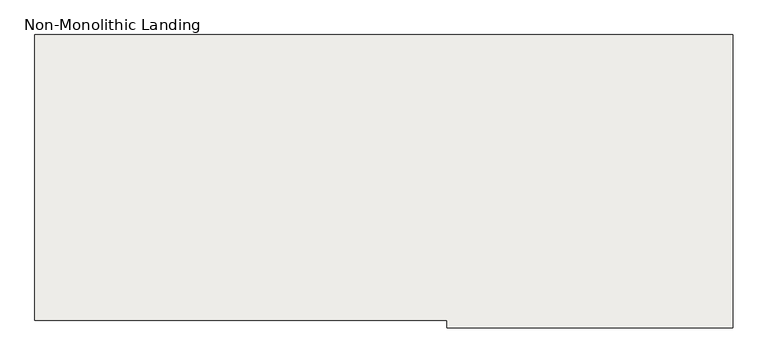
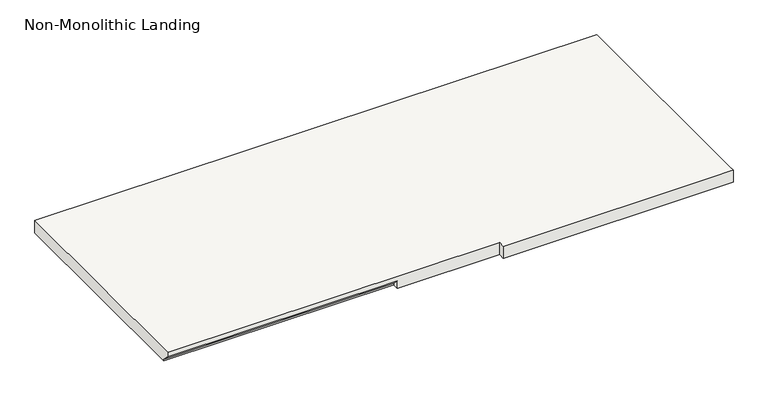
"""IFC4 building model written with IfcOpenShell, lengths in millimetres: slab geometry, Non-Monolithic Landing."""

from ifc_helpers import new_model, si_unit, origin, place, context, project, spatial, faceted_brep, source, transform, mapped, element, save


def non_monolithic_landing_f4425cc3(model_context):
    return source(origin(), model_context, "Body", "Brep", [
        faceted_brep([(-3617.4415084, -19522.1851539, 42826.2339133), (-3617.4415084, -19496.7851539, 42800.8339133), (-2703.0415084, -19496.7851539, 42800.8339133), (-2703.0415084, -19522.1851539, 42826.2339133), (-2296.6415084, -19522.1851539, 42845.2839133), (-2296.6415084, -19547.5851539, 42845.2839133), (-1382.2415084, -19547.5851539, 42845.2839133), (-1382.2415084, -19522.1851539, 42845.2839133), (-1382.2415084, -18607.7851539, 42845.2839133), (-3617.4415084, -18607.7851539, 42845.2839133), (-3617.4415084, -19522.1851539, 42845.2839133), (-2703.0415084, -19496.7851539, 42794.4839133), (-3617.4415084, -19496.7851539, 42794.4839133), (-3617.4415084, -18607.7851539, 42794.4839133), (-1382.2415084, -18607.7851539, 42794.4839133), (-1382.2415084, -19522.1851539, 42794.4839133), (-1382.2415084, -19547.5851539, 42794.4839133), (-2296.6415084, -19547.5851539, 42794.4839133), (-2296.6415084, -19522.1851539, 42794.4839133), (-2703.0415084, -19522.1851539, 42794.4839133)], [[[0, 1, 2, 3]], [[4, 5, 6, 7, 8, 9, 10]], [[11, 12, 13, 14, 15, 16, 17, 18, 19]], [[12, 11, 2, 1]], [[11, 19, 3, 2]], [[4, 10, 0, 3, 19, 18]], [[5, 4, 18, 17]], [[6, 5, 17, 16]], [[7, 6, 16, 15]], [[8, 7, 15, 14]], [[9, 8, 14, 13]], [[10, 9, 13, 12, 1, 0]]]),
    ])


if __name__ == "__main__":
    model = new_model("IFC4")
    model_context = context("Model", 3, world=origin())
    ifc_project = project(units=[si_unit("LENGTHUNIT", "METRE", prefix="MILLI")], contexts=[model_context])
    site = spatial("IfcSite", under=ifc_project)
    building = spatial("IfcBuilding", under=site)
    placement = place(None, origin())
    non_monolithic_landing_shape = non_monolithic_landing_f4425cc3(model_context)
    element("IfcSlab", 1, ObjectType="Non-Monolithic Landing", at=placement, inside=building, context=model_context, shape_type="MappedRepresentation", body=[
        mapped(non_monolithic_landing_shape, transform((0.0, 0.0, 0.0), x_axis=(1.0, 0.0, 0.0), y_axis=(0.0, 1.0, 0.0), z_axis=(0.0, 0.0, 1.0))),
    ])
    save(model, "model.ifc")
